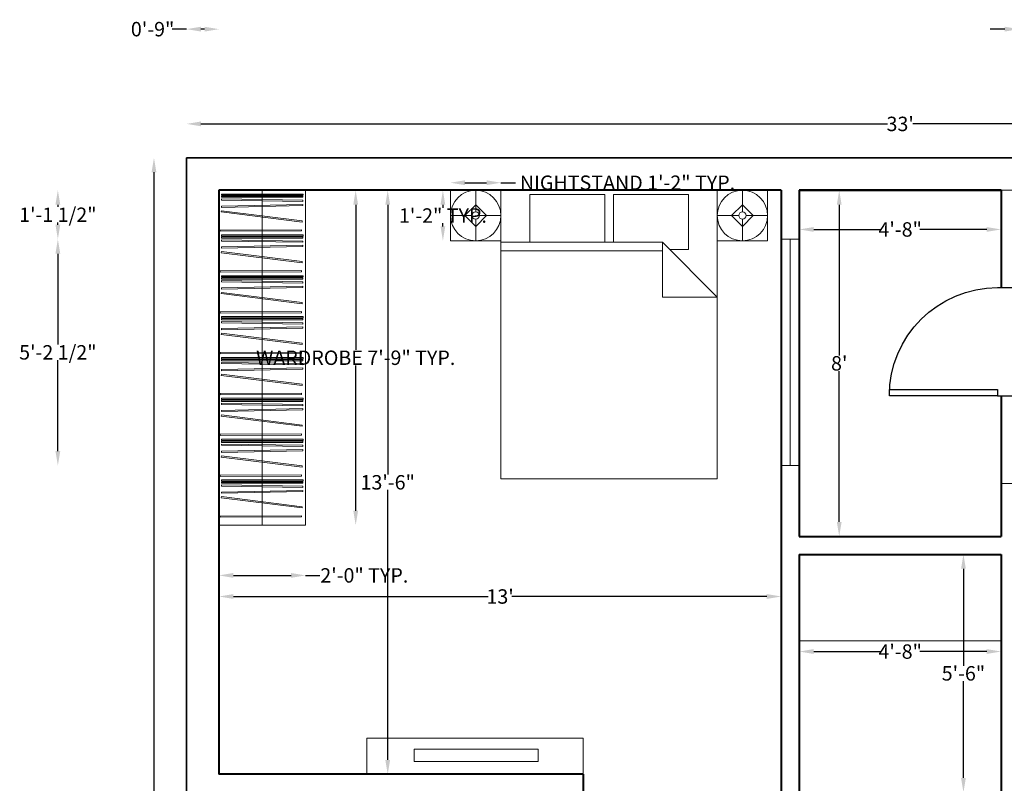
# Model space of a CAD drawing. Units: inches. Extents: x -46 to 447, y -42 to 702.
# Tile 5 of 7: x -46 to 227, y 487 to 698. Entities that reach past the tile are written whole.
import ezdxf

# ---------------------------------------------------------------- set-up
doc = ezdxf.new("R2010")
doc.units = ezdxf.units.IN
doc.header["$PDMODE"] = 3
for name, color, linetype, lineweight in [('A-ANNO-DIMS', 2, 'Continuous', 13), ('A-DOOR', 3, 'Continuous', 25), ('A-FLOR-CASE', 32, 'Continuous', 18), ('A-FURN', 8, 'Continuous', 18), ('A-GLAZ', 4, 'Continuous', 18), ('A-WALL', 7, 'Continuous', 40), ('L-WALL', 7, 'Continuous', 35)]:
    doc.layers.add(name, color=color, linetype=linetype, lineweight=lineweight)
doc.styles.get("Standard").update_dxf_attribs({"font": 'arial.ttf'})
doc.dimstyles.get("Standard").update_dxf_attribs({"dimtxt": 4, "dimasz": 4, "dimexe": 0.18, "dimexo": 0.0625, "dimgap": 0.09, "dimtad": 0, "dimtih": 1, "dimtoh": 1, "dimdec": 0, "dimzin": 0, "dimdsep": 46, "dimlunit": 3, "dimtxsty": 'Standard', "dimcen": 0.09, "dimse1": 1, "dimse2": 1, "dimadec": 0, "dimazin": 0, "dimtfac": 1, "dimtdec": 0, "dimtofl": 0, "dimtmove": 0, "dimatfit": 3, "dimfxl": 1, "dimtolj": 1, "dimtzin": 0, "dimarcsym": 0})

# ---------------------------------------------------------------- blocks, each defined once
blk = doc.blocks.new('*U3')
for p, q in [((-30, 0), (-30, -6)), ((0, 0), (0, -6))]:
    blk.add_line(p, q)
blk.add_lwpolyline([(0, 0), (0, 30), (-1.75, 30), (-1.75, 0)], close=True)
blk.add_arc((0, 0), 30, 90, 180)
blk = doc.blocks.new('Bed - Queen')
for p, q in [((0, -80.00003), (0, 0)), ((0, 0), (59.99999, 0)), ((59.99999, 0), (59.99999, -80.00003)), ((7.99999, -1.2), (28.79998, -1.2)), ((7.99999, -14.4), (7.99999, -1.2)), ((28.79998, -1.2), (28.79998, -14.4)), ((31.19999, -1.2), (51.99999, -1.2)), ((31.19999, -14.4), (31.19999, -1.2)), ((51.99999, -1.2), (51.99999, -16.4)), ((0, -14.4), (44.8, -14.4)), ((59.99999, -29.6), (44.8, -14.4)), ((44.8, -14.4), (44.8, -29.6)), ((44.8, -16.8), (0, -16.8)), ((51.99999, -16.4), (46.79936, -16.4)), ((44.8, -29.6), (59.99999, -29.6)), ((59.99999, -80.00003), (0, -80.00003))]:
    blk.add_line(p, q)
blk = doc.blocks.new('Lamp - Table')
for p, q in [((0, 7), (0, 1)), ((0, 3), (-3, 0)), ((3, 0), (0, 3)), ((-1, 0), (-7, 0)), ((-3, 0), (0, -3)), ((0, -3), (3, 0)), ((1, 0), (7, 0)), ((0, -1), (0, -7))]:
    blk.add_line(p, q)
for radius in [7, 1]:
    blk.add_circle((0, 0), radius)
blk = doc.blocks.new('*D49')
at = {"layer": 'A-ANNO-DIMS', "color": 0, "lineweight": -2, "transparency": 16777216}
for p, q in [((4, 669.42), (194.52, 669.42)), ((392, 669.42), (201.48, 669.42))]:
    blk.add_line(p, q, dxfattribs=at)
at = {"layer": 'A-ANNO-DIMS', "color": 0, "transparency": 16777216}
for points in [[(4, 670.09), (4, 668.76), (0, 669.42)], [(392, 670.09), (392, 668.76), (396, 669.42)]]:
    blk.add_solid(points, dxfattribs=at)
at = {"layer": 'Defpoints', "color": 0, "transparency": 16777216}
for p in [(396, 669.42), (0, 660), (396, 660)]:
    blk.add_point(p, dxfattribs=at)
at = {"layer": 'A-ANNO-DIMS', "color": 0, "transparency": 16777216, "insert": (198, 669.42), "char_height": 4, "attachment_point": 5}
blk.add_mtext("\\A1;33'", dxfattribs=at)
blk = doc.blocks.new('*D50')
at = {"layer": 'A-ANNO-DIMS', "color": 0, "lineweight": -2, "transparency": 16777216}
for p, q in [((-9.03, 656), (-9.03, 332.12)), ((-9.03, 4), (-9.03, 327.88))]:
    blk.add_line(p, q, dxfattribs=at)
at = {"layer": 'A-ANNO-DIMS', "color": 0, "transparency": 16777216}
for points in [[(-9.7, 656), (-8.36, 656), (-9.03, 660)], [(-9.7, 4), (-8.36, 4), (-9.03, 0)]]:
    blk.add_solid(points, dxfattribs=at)
at = {"layer": 'Defpoints', "color": 0, "transparency": 16777216}
for p in [(0, 660), (0, 0), (-9.03, 0)]:
    blk.add_point(p, dxfattribs=at)
at = {"layer": 'A-ANNO-DIMS', "color": 0, "transparency": 16777216, "insert": (-9.03, 330), "char_height": 4, "attachment_point": 5}
blk.add_mtext("\\A1;55'", dxfattribs=at)
blk = doc.blocks.new('*D69')
at = {"layer": 'A-ANNO-DIMS', "color": 0, "lineweight": -2, "transparency": 16777216}
for p, q in [((215.55, 546), (215.55, 519.13)), ((215.55, 488), (215.55, 514.87))]:
    blk.add_line(p, q, dxfattribs=at)
at = {"layer": 'A-ANNO-DIMS', "color": 0, "transparency": 16777216}
for points in [[(214.89, 546), (216.22, 546), (215.55, 550)], [(214.89, 488), (216.22, 488), (215.55, 484)]]:
    blk.add_solid(points, dxfattribs=at)
at = {"layer": 'Defpoints', "color": 0, "transparency": 16777216}
for p in [(226, 550), (215.55, 484), (226, 484)]:
    blk.add_point(p, dxfattribs=at)
at = {"layer": 'A-ANNO-DIMS', "color": 0, "transparency": 16777216, "insert": (215.55, 517), "char_height": 4, "attachment_point": 5}
blk.add_mtext('\\A1;5\'-6"', dxfattribs=at)
blk = doc.blocks.new('*D70')
at = {"layer": 'A-ANNO-DIMS', "color": 0, "lineweight": -2, "transparency": 16777216}
for p, q in [((174, 523.05), (192.51, 523.05)), ((222, 523.05), (203.49, 523.05))]:
    blk.add_line(p, q, dxfattribs=at)
at = {"layer": 'A-ANNO-DIMS', "color": 0, "transparency": 16777216}
for points in [[(174, 523.72), (174, 522.38), (170, 523.05)], [(222, 523.72), (222, 522.38), (226, 523.05)]]:
    blk.add_solid(points, dxfattribs=at)
at = {"layer": 'Defpoints', "color": 0, "transparency": 16777216}
for p in [(170, 550), (226, 550), (226, 523.05)]:
    blk.add_point(p, dxfattribs=at)
at = {"layer": 'A-ANNO-DIMS', "color": 0, "transparency": 16777216, "insert": (198, 523.05), "char_height": 4, "attachment_point": 5}
blk.add_mtext('\\A1;4\'-8"', dxfattribs=at)
blk = doc.blocks.new('*D73')
at = {"layer": 'A-ANNO-DIMS', "color": 0, "lineweight": -2, "transparency": 16777216}
for p, q in [((55.82, 647), (55.82, 572.13)), ((55.82, 493), (55.82, 567.87))]:
    blk.add_line(p, q, dxfattribs=at)
at = {"layer": 'A-ANNO-DIMS', "color": 0, "transparency": 16777216}
for points in [[(55.15, 647), (56.49, 647), (55.82, 651)], [(55.15, 493), (56.49, 493), (55.82, 489)]]:
    blk.add_solid(points, dxfattribs=at)
at = {"layer": 'Defpoints', "color": 0, "transparency": 16777216}
for p in [(9, 651), (9, 489), (55.82, 489)]:
    blk.add_point(p, dxfattribs=at)
at = {"layer": 'A-ANNO-DIMS', "color": 0, "transparency": 16777216, "insert": (55.82, 570), "char_height": 4, "attachment_point": 5}
blk.add_mtext('\\A1;13\'-6"', dxfattribs=at)
blk = doc.blocks.new('*D74')
at = {"layer": 'A-ANNO-DIMS', "color": 0, "lineweight": -2, "transparency": 16777216}
for p, q in [((13, 538.32), (83.7, 538.32)), ((161, 538.32), (90.3, 538.32))]:
    blk.add_line(p, q, dxfattribs=at)
at = {"layer": 'A-ANNO-DIMS', "color": 0, "transparency": 16777216}
for points in [[(13, 538.99), (13, 537.65), (9, 538.32)], [(161, 538.99), (161, 537.65), (165, 538.32)]]:
    blk.add_solid(points, dxfattribs=at)
at = {"layer": 'Defpoints', "color": 0, "transparency": 16777216}
for p in [(9, 651), (165, 651), (9, 538.32)]:
    blk.add_point(p, dxfattribs=at)
at = {"layer": 'A-ANNO-DIMS', "color": 0, "transparency": 16777216, "insert": (87, 538.32), "char_height": 4, "attachment_point": 5}
blk.add_mtext("\\A1;13'", dxfattribs=at)
blk = doc.blocks.new('*D77')
at = {"layer": 'A-ANNO-DIMS', "color": 0, "lineweight": -2, "transparency": 16777216}
for p, q in [((174, 640.14), (192.51, 640.14)), ((222, 640.14), (203.49, 640.14))]:
    blk.add_line(p, q, dxfattribs=at)
at = {"layer": 'A-ANNO-DIMS', "color": 0, "transparency": 16777216}
for points in [[(174, 640.81), (174, 639.48), (170, 640.14)], [(222, 640.81), (222, 639.48), (226, 640.14)]]:
    blk.add_solid(points, dxfattribs=at)
at = {"layer": 'Defpoints', "color": 0, "transparency": 16777216}
for p in [(170, 651), (226, 651), (226, 640.14)]:
    blk.add_point(p, dxfattribs=at)
at = {"layer": 'A-ANNO-DIMS', "color": 0, "transparency": 16777216, "insert": (198, 640.14), "char_height": 4, "attachment_point": 5}
blk.add_mtext('\\A1;4\'-8"', dxfattribs=at)
blk = doc.blocks.new('*D78')
at = {"layer": 'A-ANNO-DIMS', "color": 0, "lineweight": -2, "transparency": 16777216}
for p, q in [((181.09, 647), (181.09, 605.13)), ((181.09, 559), (181.09, 600.87))]:
    blk.add_line(p, q, dxfattribs=at)
at = {"layer": 'A-ANNO-DIMS', "color": 0, "transparency": 16777216}
for points in [[(180.42, 647), (181.76, 647), (181.09, 651)], [(180.42, 559), (181.76, 559), (181.09, 555)]]:
    blk.add_solid(points, dxfattribs=at)
at = {"layer": 'Defpoints', "color": 0, "transparency": 16777216}
for p in [(170, 651), (170, 555), (181.09, 555)]:
    blk.add_point(p, dxfattribs=at)
at = {"layer": 'A-ANNO-DIMS', "color": 0, "transparency": 16777216, "insert": (181.09, 603), "char_height": 4, "attachment_point": 5}
blk.add_mtext("\\A1;8'", dxfattribs=at)
blk = doc.blocks.new('WARDROBE-93X24')
for p, q in [((12, -92.9), (12, 0)), ((24, 0), (24, -92.9)), ((24, -92.9), (0, -92.9))]:
    blk.add_line(p, q)
for points in [[(0.7, -1.6), (23.3, -1.6), (23.3, -1.95), (0.7, -1.95)], [(23.3, -3.1), (0.7, -2.75), (0.7, -2.4), (23.3, -2.75)], [(0.72, -1.03), (23.33, -1.03), (23.33, -1.38), (0.72, -1.38)], [(23.3, -4.26), (0.7, -4.73), (0.7, -4.38), (23.3, -3.91)], [(23.09, -8.46), (0.66, -5.66), (0.61, -6), (23.04, -8.81)], [(22.92, -11.29), (0.31, -11.38), (0.31, -11.03), (22.91, -10.94)], [(0.7, -12.93), (23.3, -12.93), (23.3, -13.28), (0.7, -13.28)], [(0.72, -12.37), (23.33, -12.37), (23.33, -12.72), (0.72, -12.72)], [(23.3, -14.43), (0.7, -14.08), (0.7, -13.73), (23.3, -14.08)], [(23.3, -15.59), (0.7, -16.06), (0.7, -15.71), (23.3, -15.24)], [(23.09, -19.79), (0.66, -16.99), (0.61, -17.34), (23.04, -20.14)], [(22.92, -22.62), (0.31, -22.71), (0.31, -22.36), (22.91, -22.27)], [(0.7, -24.26), (23.3, -24.26), (23.3, -24.61), (0.7, -24.61)], [(0.72, -23.7), (23.33, -23.7), (23.33, -24.05), (0.72, -24.05)], [(23.3, -25.77), (0.7, -25.41), (0.7, -25.06), (23.3, -25.41)], [(23.3, -26.93), (0.7, -27.39), (0.7, -27.04), (23.3, -26.57)], [(23.09, -31.12), (0.66, -28.32), (0.61, -28.67), (23.04, -31.47)], [(22.92, -33.95), (0.31, -34.04), (0.31, -33.69), (22.91, -33.6)], [(0.72, -35.03), (23.33, -35.03), (23.33, -35.38), (0.72, -35.38)], [(0.7, -35.59), (23.3, -35.59), (23.3, -35.94), (0.7, -35.94)], [(23.3, -37.1), (0.7, -36.75), (0.7, -36.39), (23.3, -36.75)], [(23.3, -38.26), (0.7, -38.72), (0.7, -38.37), (23.3, -37.91)], [(23.09, -42.45), (0.66, -39.65), (0.61, -40), (23.04, -42.8)], [(22.92, -45.28), (0.31, -45.37), (0.31, -45.02), (22.91, -44.93)], [(0.72, -46.36), (23.33, -46.36), (23.33, -46.71), (0.72, -46.71)], [(0.7, -46.92), (23.3, -46.92), (23.3, -47.27), (0.7, -47.27)], [(23.3, -48.43), (0.7, -48.08), (0.7, -47.73), (23.3, -48.08)], [(23.09, -53.79), (0.66, -50.98), (0.61, -51.33), (23.04, -54.13)], [(23.3, -49.59), (0.7, -50.05), (0.7, -49.7), (23.3, -49.24)], [(22.92, -56.61), (0.31, -56.7), (0.31, -56.35), (22.91, -56.26)], [(0.7, -58.25), (23.3, -58.25), (23.3, -58.6), (0.7, -58.6)], [(23.3, -59.76), (0.7, -59.41), (0.7, -59.06), (23.3, -59.41)], [(0.72, -57.69), (23.33, -57.69), (23.33, -58.04), (0.72, -58.04)], [(23.09, -65.12), (0.66, -62.31), (0.61, -62.66), (23.04, -65.47)], [(23.3, -60.92), (0.7, -61.39), (0.7, -61.04), (23.3, -60.57)], [(22.92, -67.95), (0.31, -68.04), (0.31, -67.68), (22.91, -67.59)], [(0.7, -69.59), (23.3, -69.59), (23.3, -69.94), (0.7, -69.94)], [(23.3, -71.09), (0.7, -70.74), (0.7, -70.39), (23.3, -70.74)], [(0.72, -69.02), (23.33, -69.02), (23.33, -69.37), (0.72, -69.37)], [(23.09, -76.45), (0.66, -73.64), (0.61, -73.99), (23.04, -76.8)], [(23.3, -72.25), (0.7, -72.72), (0.7, -72.37), (23.3, -71.9)], [(22.92, -79.28), (0.31, -79.37), (0.31, -79.02), (22.91, -78.93)], [(0.7, -80.92), (23.3, -80.92), (23.3, -81.27), (0.7, -81.27)], [(23.3, -82.42), (0.7, -82.07), (0.7, -81.72), (23.3, -82.07)], [(0.72, -80.35), (23.33, -80.35), (23.33, -80.71), (0.72, -80.71)], [(23.3, -83.58), (0.7, -84.05), (0.7, -83.7), (23.3, -83.23)], [(23.09, -87.78), (0.66, -84.98), (0.61, -85.32), (23.04, -88.13)], [(22.92, -90.61), (0.31, -90.7), (0.31, -90.35), (22.91, -90.26)]]:
    blk.add_lwpolyline(points, close=True)
blk = doc.blocks.new('MEDIA-CONSOLE-60')
for points in [[(60, 0), (0, 0), (0, 10), (60, 10)], [(13.13, 6.99), (47.53, 6.99), (47.53, 3.54), (13.13, 3.54)]]:
    blk.add_lwpolyline(points, close=True)
blk = doc.blocks.new('NIGHTSTAND-14')
blk.add_lwpolyline([(0, 0), (0, -14.000002), (14.000002, -14.000002), (14.000002, 0)], close=True)
blk = doc.blocks.new('*D86')
at = {"layer": 'A-ANNO-DIMS', "color": 0, "lineweight": -2, "transparency": 16777216}
for p, q in [((46.93, 647), (46.93, 606.71)), ((46.93, 562.1), (46.93, 602.39))]:
    blk.add_line(p, q, dxfattribs=at)
at = {"layer": 'A-ANNO-DIMS', "color": 0, "transparency": 16777216}
for points in [[(46.27, 647), (47.6, 647), (46.93, 651)], [(46.27, 562.1), (47.6, 562.1), (46.93, 558.1)]]:
    blk.add_solid(points, dxfattribs=at)
at = {"layer": 'Defpoints', "color": 0, "transparency": 16777216}
for p in [(33, 651), (46.93, 651), (33, 558.1)]:
    blk.add_point(p, dxfattribs=at)
at = {"layer": 'A-ANNO-DIMS', "color": 0, "transparency": 16777216, "insert": (46.93, 604.55), "char_height": 4, "attachment_point": 5}
blk.add_mtext('\\A1;WARDROBE 7\'-9" TYP.', dxfattribs=at)
blk = doc.blocks.new('*D87')
at = {"layer": 'A-ANNO-DIMS', "color": 0, "lineweight": -2, "transparency": 16777216}
for p, q in [((13, 544.17), (29, 544.17)), ((33, 544.17), (37, 544.17))]:
    blk.add_line(p, q, dxfattribs=at)
at = {"layer": 'A-ANNO-DIMS', "color": 0, "transparency": 16777216}
for points in [[(13, 544.84), (13, 543.5), (9, 544.17)], [(29, 544.84), (29, 543.5), (33, 544.17)]]:
    blk.add_solid(points, dxfattribs=at)
at = {"layer": 'Defpoints', "color": 0, "transparency": 16777216}
for p in [(9, 558.1), (33, 558.1), (33, 544.17)]:
    blk.add_point(p, dxfattribs=at)
at = {"layer": 'A-ANNO-DIMS', "color": 0, "transparency": 16777216, "insert": (49.32, 544.17), "char_height": 4, "attachment_point": 5}
blk.add_mtext('\\A1;2\'-0" TYP.', dxfattribs=at)
blk = doc.blocks.new('*D90')
at = {"layer": 'A-ANNO-DIMS', "color": 0, "lineweight": -2, "transparency": 16777216}
for p, q in [((77.23, 653.1), (83.23, 653.1)), ((87.23, 653.1), (91.23, 653.1))]:
    blk.add_line(p, q, dxfattribs=at)
at = {"layer": 'A-ANNO-DIMS', "color": 0, "transparency": 16777216}
for points in [[(77.23, 653.77), (77.23, 652.43), (73.23, 653.1)], [(83.23, 653.77), (83.23, 652.43), (87.23, 653.1)]]:
    blk.add_solid(points, dxfattribs=at)
at = {"layer": 'Defpoints', "color": 0, "transparency": 16777216}
for p in [(87.23, 653.1), (73.23, 651), (87.23, 651)]:
    blk.add_point(p, dxfattribs=at)
at = {"layer": 'A-ANNO-DIMS', "color": 0, "transparency": 16777216, "insert": (122.35, 653.1), "char_height": 4, "attachment_point": 5}
blk.add_mtext('\\A1;NIGHTSTAND 1\'-2" TYP.', dxfattribs=at)
blk = doc.blocks.new('*D91')
at = {"layer": 'A-ANNO-DIMS', "color": 0, "lineweight": -2, "transparency": 16777216}
for p, q in [((71.13, 647), (71.13, 646.1)), ((71.13, 641), (71.13, 641.9))]:
    blk.add_line(p, q, dxfattribs=at)
at = {"layer": 'A-ANNO-DIMS', "color": 0, "transparency": 16777216}
for points in [[(70.46, 647), (71.79, 647), (71.13, 651)], [(70.46, 641), (71.79, 641), (71.13, 637)]]:
    blk.add_solid(points, dxfattribs=at)
at = {"layer": 'Defpoints', "color": 0, "transparency": 16777216}
for p in [(71.13, 651), (73.23, 651), (73.23, 637)]:
    blk.add_point(p, dxfattribs=at)
at = {"layer": 'A-ANNO-DIMS', "color": 0, "transparency": 16777216, "insert": (71.13, 644), "char_height": 4, "attachment_point": 5}
blk.add_mtext('\\A1;1\'-2" TYP.', dxfattribs=at)
blk = doc.blocks.new('*D130')
at = {"layer": 'A-ANNO-DIMS', "color": 0, "lineweight": -2, "transparency": 16777216}
for p, q in [((0, 695.7), (-4, 695.7)), ((5, 695.7), (4, 695.7))]:
    blk.add_line(p, q, dxfattribs=at)
at = {"layer": 'A-ANNO-DIMS', "color": 0, "transparency": 16777216}
for points in [[(4, 696.37), (4, 695.03), (0, 695.7)], [(5, 696.37), (5, 695.03), (9, 695.7)]]:
    blk.add_solid(points, dxfattribs=at)
at = {"layer": 'Defpoints', "color": 0, "transparency": 16777216}
for p in [(0, 695.7), (0, 446.66), (9, 446.66)]:
    blk.add_point(p, dxfattribs=at)
at = {"layer": 'A-ANNO-DIMS', "color": 0, "transparency": 16777216, "insert": (-9.41, 695.7), "char_height": 4, "attachment_point": 5}
blk.add_mtext('\\A1;0\'-9"', dxfattribs=at)
blk = doc.blocks.new('*D139')
at = {"layer": 'A-ANNO-DIMS', "color": 0, "lineweight": -2, "transparency": 16777216}
for p, q in [((431.7, 590), (431.7, 584.01)), ((431.7, 573.71), (431.7, 579.7))]:
    blk.add_line(p, q, dxfattribs=at)
at = {"layer": 'A-ANNO-DIMS', "color": 0, "transparency": 16777216}
for points in [[(431.03, 590), (432.37, 590), (431.7, 594)], [(431.03, 573.71), (432.37, 573.71), (431.7, 569.71)]]:
    blk.add_solid(points, dxfattribs=at)
at = {"layer": 'Defpoints', "color": 0, "transparency": 16777216}
for p in [(226, 594), (431.7, 594), (226, 569.71)]:
    blk.add_point(p, dxfattribs=at)
at = {"layer": 'A-ANNO-DIMS', "color": 0, "transparency": 16777216, "insert": (431.7, 581.85), "char_height": 4, "attachment_point": 5}
blk.add_mtext('\\A1;2\'-0 1/2"', dxfattribs=at)
blk = doc.blocks.new('*D140')
at = {"layer": 'A-ANNO-DIMS', "color": 0, "lineweight": -2, "transparency": 16777216}
for p, q in [((-35.7, 633.42), (-35.7, 608.21)), ((-35.7, 578.68), (-35.7, 603.89))]:
    blk.add_line(p, q, dxfattribs=at)
at = {"layer": 'A-ANNO-DIMS', "color": 0, "transparency": 16777216}
for points in [[(-36.37, 633.42), (-35.03, 633.42), (-35.7, 637.42)], [(-36.37, 578.68), (-35.03, 578.68), (-35.7, 574.68)]]:
    blk.add_solid(points, dxfattribs=at)
at = {"layer": 'Defpoints', "color": 0, "transparency": 16777216}
for p in [(-35.7, 637.42), (170, 637.42), (170, 574.68)]:
    blk.add_point(p, dxfattribs=at)
at = {"layer": 'A-ANNO-DIMS', "color": 0, "transparency": 16777216, "insert": (-35.7, 606.05), "char_height": 4, "attachment_point": 5}
blk.add_mtext('\\A1;5\'-2 1/2"', dxfattribs=at)
blk = doc.blocks.new('*D141')
at = {"layer": 'A-ANNO-DIMS', "color": 0, "lineweight": -2, "transparency": 16777216}
for p, q in [((-35.7, 647), (-35.7, 646.37)), ((-35.7, 641.42), (-35.7, 642.05))]:
    blk.add_line(p, q, dxfattribs=at)
at = {"layer": 'A-ANNO-DIMS', "color": 0, "transparency": 16777216}
for points in [[(-36.37, 647), (-35.03, 647), (-35.7, 651)], [(-36.37, 641.42), (-35.03, 641.42), (-35.7, 637.42)]]:
    blk.add_solid(points, dxfattribs=at)
at = {"layer": 'Defpoints', "color": 0, "transparency": 16777216}
for p in [(-35.7, 651), (170, 651), (170, 637.42)]:
    blk.add_point(p, dxfattribs=at)
at = {"layer": 'A-ANNO-DIMS', "color": 0, "transparency": 16777216, "insert": (-35.7, 644.21), "char_height": 4, "attachment_point": 5}
blk.add_mtext('\\A1;1\'-1 1/2"', dxfattribs=at)
blk = doc.blocks.new('*D148')
at = {"layer": 'A-ANNO-DIMS', "color": 0, "lineweight": -2, "transparency": 16777216}
for p, q in [((227, 695.7), (223, 695.7)), ((238.24, 695.7), (242.24, 695.7))]:
    blk.add_line(p, q, dxfattribs=at)
at = {"layer": 'A-ANNO-DIMS', "color": 0, "transparency": 16777216}
for points in [[(227, 696.37), (227, 695.03), (231, 695.7)], [(238.24, 696.37), (238.24, 695.03), (234.24, 695.7)]]:
    blk.add_solid(points, dxfattribs=at)
at = {"layer": 'Defpoints', "color": 0, "transparency": 16777216}
for p in [(234.24, 695.7), (231, 319), (234.24, 319)]:
    blk.add_point(p, dxfattribs=at)
at = {"layer": 'A-ANNO-DIMS', "color": 0, "transparency": 16777216, "insert": (247.64, 695.7), "char_height": 4, "attachment_point": 5}
blk.add_mtext('\\A1;0\'-3"', dxfattribs=at)

msp = doc.modelspace()

# ---------------------------------------------------------------- linework, layer by layer
at = {"layer": 'A-FLOR-CASE'}
msp.add_line((170, 526), (226, 526), dxfattribs=at)
at = {"layer": 'A-GLAZ'}
for p, q in [((226, 651), (231, 651)), ((165, 637.42), (170, 637.42)), ((167.5, 637.42), (167.5, 574.68)), ((231, 624), (226, 624)), ((165, 574.68), (170, 574.68)), ((226, 569.71), (231, 569.71))]:
    msp.add_line(p, q, dxfattribs=at)
at = {"layer": 'A-WALL'}
for p, q in [((9, 651), (9, 489)), ((165, 651), (9, 651)), ((165, 651), (165, 468.57)), ((170, 651), (170, 555)), ((170, 651), (226, 651)), ((226, 651), (170, 651)), ((226, 651), (226, 624)), ((226, 594), (226, 555)), ((170, 555), (226, 555)), ((170, 550), (226, 550)), ((170, 550), (170, 468.57)), ((226, 550), (226, 484)), ((110, 489), (9, 489)), ((110, 489), (110, 483.23))]:
    msp.add_line(p, q, dxfattribs=at)
at = {"layer": 'L-WALL'}
msp.add_lwpolyline([(222, 0), (396, 0), (396, 660), (0, 660), (0, 0), (17.93, 0)], dxfattribs=at)

# ---------------------------------------------------------------- block references
at = {"layer": 'A-DOOR', "xscale": -1, "rotation": 90}
msp.add_blockref('*U3', (225, 594), dxfattribs=at)
at = {"layer": 'A-FLOR-CASE'}
for name, p in [('WARDROBE-93X24', (9, 651)), ('MEDIA-CONSOLE-60', (50, 489))]:
    msp.add_blockref(name, p, dxfattribs=at)
at = {"layer": 'A-FURN'}
for name, p in [('Lamp - Table', (80.23, 644)), ('NIGHTSTAND-14', (73.23, 651)), ('Bed - Queen', (87.23, 651))]:
    msp.add_blockref(name, p, dxfattribs=at)
at = {"layer": 'A-FURN', "xscale": -1}
msp.add_blockref('Lamp - Table', (154.23, 644), dxfattribs=at)
at = {"layer": 'A-FURN', "rotation": 270.0000000000002}
msp.add_blockref('NIGHTSTAND-14', (161.23, 651), dxfattribs=at)

# ---------------------------------------------------------------- dimensions: what is measured, and where the dimension line sits
at = {"layer": 'A-ANNO-DIMS'}
for base, p1, p2, override, picture, middle in [((0, 695.7), (9, 446.66), (0, 446.66), {"dimdec": 1, "dimlfac": 1, "dimrnd": 0, "dimzin": 1, "dimdsep": 46, "dimlunit": 4, "dimfrac": 2}, '*D130', (-9.41, 695.7)), ((234.24, 695.7), (231, 319), (234.24, 319), {"dimdec": 1, "dimlfac": 1, "dimrnd": 0, "dimzin": 1, "dimdsep": 46, "dimlunit": 4, "dimfrac": 2}, '*D148', (247.64, 695.7)), ((396, 669.42), (0, 660), (396, 660), {"dimclrd": 0, "dimclre": 0, "dimclrt": 0}, '*D49', (198, 669.42)), ((9, 538.32), (165, 651), (9, 651), {"dimclrd": 0, "dimclre": 0, "dimclrt": 0}, '*D74', (87, 538.32)), ((226, 640.14), (170, 651), (226, 651), {"dimclrd": 0, "dimclre": 0, "dimclrt": 0}, '*D77', (198, 640.14)), ((226, 523.05), (170, 550), (226, 550), {"dimclrd": 0, "dimclre": 0, "dimclrt": 0}, '*D70', (198, 523.05))]:
    dim = msp.add_linear_dim(base=base, p1=p1, p2=p2, dimstyle='Standard', override=override, dxfattribs=at)
    dim.commit()
    dim.dimension.update_dxf_attribs({"geometry": picture, "text_midpoint": middle})
for base, p1, p2, text, picture, middle in [((87.23, 653.1), (73.23, 651), (87.23, 651), 'NIGHTSTAND <> TYP.', '*D90', (122.35, 653.1)), ((33, 544.17), (9, 558.1), (33, 558.1), '<> TYP.', '*D87', (49.32, 544.17))]:
    dim = msp.add_linear_dim(base=base, p1=p1, p2=p2, text=text, dimstyle='Standard', override={"dimdec": 1, "dimlfac": 1, "dimrnd": 0, "dimzin": 1, "dimdsep": 46, "dimlunit": 4, "dimfrac": 2}, dxfattribs=at)
    dim.commit()
    dim.dimension.update_dxf_attribs({"geometry": picture, "text_midpoint": middle})
for base, p1, p2, override, picture, middle in [((-9.03, 0), (0, 660), (0, 0), {"dimclrd": 0, "dimclre": 0, "dimclrt": 0}, '*D50', (-9.03, 330)), ((-35.7, 651), (170, 637.42), (170, 651), {"dimdec": 1, "dimlfac": 1, "dimrnd": 0, "dimzin": 1, "dimdsep": 46, "dimlunit": 4, "dimfrac": 2}, '*D141', (-35.7, 644.21)), ((55.82, 489), (9, 651), (9, 489), {"dimclrd": 0, "dimclre": 0, "dimclrt": 0}, '*D73', (55.82, 570)), ((181.09, 555), (170, 651), (170, 555), {"dimclrd": 0, "dimclre": 0, "dimclrt": 0}, '*D78', (181.09, 603)), ((-35.7, 637.42), (170, 574.68), (170, 637.42), {"dimdec": 1, "dimlfac": 1, "dimrnd": 0, "dimzin": 1, "dimdsep": 46, "dimlunit": 4, "dimfrac": 2}, '*D140', (-35.7, 606.05)), ((431.7, 594), (226, 569.71), (226, 594), {"dimdec": 1, "dimlfac": 1, "dimrnd": 0, "dimzin": 1, "dimdsep": 46, "dimlunit": 4, "dimfrac": 2}, '*D139', (431.7, 581.85)), ((215.55, 484), (226, 550), (226, 484), {"dimclrd": 0, "dimclre": 0, "dimclrt": 0}, '*D69', (215.55, 517))]:
    dim = msp.add_linear_dim(base=base, p1=p1, p2=p2, angle=90, dimstyle='Standard', override=override, dxfattribs=at)
    dim.commit()
    dim.dimension.update_dxf_attribs({"geometry": picture, "text_midpoint": middle})
for base, p1, p2, text, picture, middle in [((46.93, 651), (33, 558.1), (33, 651), 'WARDROBE <> TYP.', '*D86', (46.93, 604.55)), ((71.13, 651), (73.23, 637), (73.23, 651), '<> TYP.', '*D91', (71.13, 644))]:
    dim = msp.add_linear_dim(base=base, p1=p1, p2=p2, angle=90, text=text, dimstyle='Standard', override={"dimdec": 1, "dimlfac": 1, "dimrnd": 0, "dimzin": 1, "dimdsep": 46, "dimlunit": 4, "dimfrac": 2}, dxfattribs=at)
    dim.commit()
    dim.dimension.update_dxf_attribs({"geometry": picture, "text_midpoint": middle})

doc.saveas('drawing.dxf')
